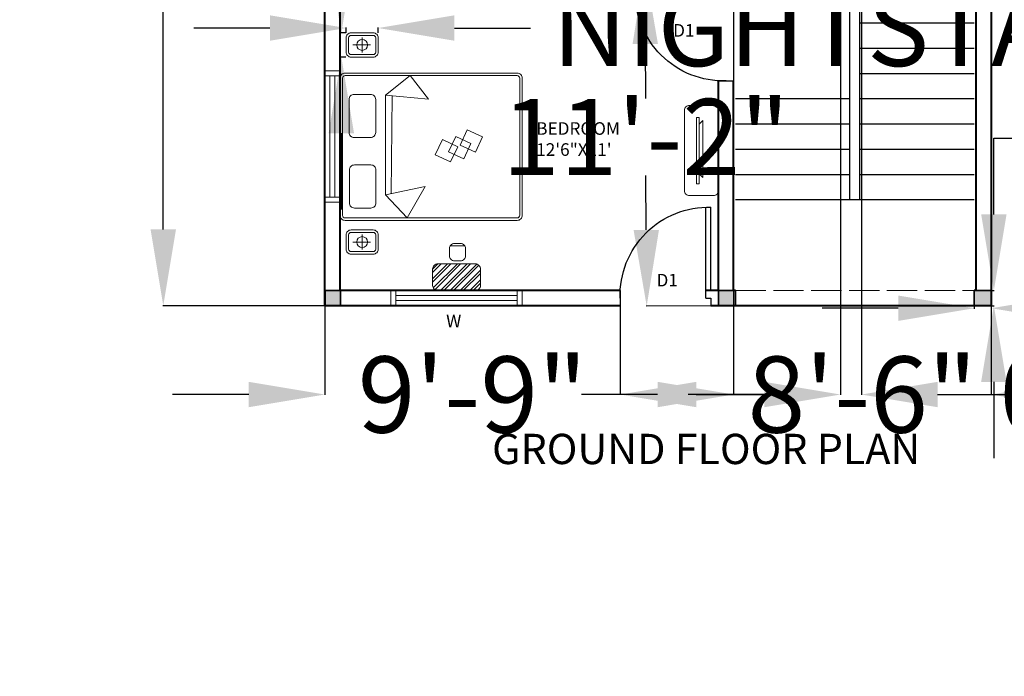
# Model space of a CAD drawing. Units: inches. Extents: x 7323 to 9737, y 2037 to 3322.
# Tile 1 of 19: x 8530 to 8921, y 2037 to 2297. Entities that reach past the tile are written whole.
import ezdxf

# ---------------------------------------------------------------- set-up
doc = ezdxf.new("R2010")
doc.units = ezdxf.units.IN
doc.header["$MEASUREMENT"] = 0
doc.linetypes.add('ACAD_ISO02W100', pattern=[15, 12, -3])
for name, color, linetype, lineweight in [('A-ANNO-DIMS', 2, 'Continuous', 18), ('A-ANNO-TEXT', 7, 'Continuous', 25), ('A-AREA-IDEN', 7, 'Continuous', 18), ('A-COLS', 1, 'Continuous', 35), ('A-DOOR', 4, 'Continuous', 25), ('A-FLOR-STRS', 7, 'Continuous', 25), ('A-FLOR-STRS-HIDN', 7, 'ACAD_ISO02W100', 18), ('A-FURN', 8, 'Continuous', 18), ('A-FURN-PATT', 252, 'Continuous', 13), ('A-GLAZ', 4, 'Continuous', 18), ('A-WALL', 7, 'Continuous', 40)]:
    doc.layers.add(name, color=color, linetype=linetype, lineweight=lineweight)
doc.layers.add('A-COLS-PATT', color=18, linetype='Continuous', lineweight=13, true_color=0x000000)
doc.styles.get("Standard").update_dxf_attribs({"font": 'arial.ttf'})
doc.dimstyles.get("Standard").update_dxf_attribs({"dimtxt": 30.18, "dimasz": 30.18, "dimexe": 0.18, "dimexo": 0.0625, "dimgap": 0.09, "dimtad": 0, "dimtih": 1, "dimtoh": 1, "dimdec": 0, "dimzin": 0, "dimdsep": 46, "dimlunit": 3, "dimtxsty": 'Standard', "dimcen": 0.09, "dimadec": 0, "dimazin": 0, "dimtfac": 1, "dimtdec": 0, "dimtofl": 0, "dimtmove": 0, "dimatfit": 3, "dimfxl": 1, "dimtolj": 1, "dimtzin": 0, "dimarcsym": 0})

# ---------------------------------------------------------------- blocks, each defined once
blk = doc.blocks.new('WIN-48')
for p, q in [((0, 0), (0, 6)), ((2, 0), (2, 6)), ((2, 4), (50, 4)), ((50, 0), (50, 6)), ((52, 0), (52, 6)), ((2, 2), (50, 2))]:
    blk.add_line(p, q)
blk = doc.blocks.new('STAIR-RETURN-FLIGHT')
for p, q in [((45.32, 110), (94.63, 110)), ((45.32, 0), (45.32, 110)), ((49.32, 0), (49.32, 110)), ((49.32, 100), (94.63, 100)), ((49.32, 90), (94.63, 90)), ((49.32, 80), (94.63, 80)), ((49.32, 70), (94.63, 70)), ((49.32, 60), (94.63, 60)), ((49.32, 50), (94.63, 50)), ((0, 40), (45.32, 40)), ((49.32, 40), (94.63, 40)), ((0, 30), (45.32, 30)), ((49.32, 30), (94.63, 30)), ((0, 20), (45.32, 20)), ((49.32, 20), (94.63, 20)), ((0, 10), (45.32, 10)), ((49.32, 10), (94.63, 10)), ((0, 0), (94.63, 0))]:
    blk.add_line(p, q)
blk = doc.blocks.new('DOOR-36')
for p, q in [((33.01, 39), (39.01, 39)), ((36.01, 5), (0.01, 5)), ((36.01, 5), (36.01, 3)), ((33.01, 3), (0.01, 3)), ((36.01, 3), (39.01, 3)), ((33.01, 0), (39.01, 0))]:
    blk.add_line(p, q)
blk.add_arc((35.01, 4), 35.01, 88.3634, 181.6366)
blk = doc.blocks.new('MEDIA-CONSOLE')
for p, q in [((5.81, 28.29), (7.29, 29.79)), ((7.29, 29.79), (7.29, 7.16)), ((7.29, 7.16), (5.81, 8.58))]:
    blk.add_line(p, q)
blk.add_lwpolyline([(13.51, 33.75, 0.414214), (11.51, 35.75), (2, 35.75, 0.414214), (0, 33.75), (0, 2, 0.414214), (2, 0), (11.51, 0, 0.414214), (13.51, 2)], format="xyb", close=True)
blk.add_lwpolyline([(5.81, 30.96), (5.81, 30.96), (4.8, 30.96), (4.8, 30.96), (4.8, 4.61), (4.8, 4.61), (5.81, 4.61), (5.81, 4.61)], close=True)
blk = doc.blocks.new('NIGHTSTAND-COMPACT')
for p, q in [((2.65, 4.81), (9.72, 4.81)), ((6.36, 7.75), (6.36, 1.85))]:
    blk.add_line(p, q)
for points in [[(0, 7.61, -0.414214), (2, 9.61), (10.71, 9.61, -0.414214), (12.71, 7.61), (12.71, 2, -0.414214), (10.71, 0), (2, 0, -0.414214), (0, 2)], [(1, 7.61, -0.414214), (2, 8.61), (10.71, 8.61, -0.414214), (11.71, 7.61), (11.71, 2, -0.414214), (10.71, 1), (2, 1, -0.414214), (1, 2)]]:
    blk.add_lwpolyline(points, format="xyb", close=True)
blk.add_circle((6.36, 4.81), 2.16)
blk = doc.blocks.new('COL-PLAN-6IN')
blk.add_lwpolyline([(0, 6), (0, 6), (6.06, 6), (6.06, 6), (6.06, 0), (6.06, 0), (0, 0), (0, 0)], close=True)
blk = doc.blocks.new('COL-STAIR-END')
blk.add_lwpolyline([(0, 6), (6.74, 6), (6.74, 0), (0, 0)], close=True)
blk = doc.blocks.new('*D43')
at = {"layer": 'A-ANNO-DIMS', "color": 0, "lineweight": -2, "transparency": 16777216}
for p, q in [((9108.94, 2438.75), (9108.94, 2468.93)), ((9104.01, 2408.57), (9109.12, 2408.57)), ((9104.01, 2375.3), (9109.12, 2375.3)), ((9108.94, 2345.12), (9108.94, 2314.94))]:
    blk.add_line(p, q, dxfattribs=at)
at = {"layer": 'A-ANNO-DIMS', "color": 0, "transparency": 16777216}
for points in [[(9103.91, 2438.75), (9113.97, 2438.75), (9108.94, 2408.57)], [(9103.91, 2345.12), (9113.97, 2345.12), (9108.94, 2375.3)]]:
    blk.add_solid(points, dxfattribs=at)
at = {"layer": 'Defpoints', "color": 0, "transparency": 16777216}
for p in [(9103.95, 2408.57), (9108.94, 2408.57), (9103.95, 2375.3)]:
    blk.add_point(p, dxfattribs=at)
at = {"layer": 'A-ANNO-DIMS', "color": 0, "transparency": 16777216, "insert": (9108.94, 2391.93), "char_height": 30.18, "attachment_point": 5}
blk.add_mtext('\\A1;BATH DOOR 2\'-9 1/2" TYP.', dxfattribs=at)
blk = doc.blocks.new('*D49')
at = {"layer": 'A-ANNO-DIMS', "color": 0, "lineweight": -2, "transparency": 16777216}
for p, q in [((8878.59, 2182.85), (8848.41, 2182.85)), ((8908.77, 2183.8), (8908.77, 2182.67)), ((8915.5, 2183.8), (8915.5, 2182.67)), ((8945.68, 2182.85), (8975.86, 2182.85))]:
    blk.add_line(p, q, dxfattribs=at)
at = {"layer": 'A-ANNO-DIMS', "color": 0, "transparency": 16777216}
for points in [[(8878.59, 2187.88), (8878.59, 2177.82), (8908.77, 2182.85)], [(8945.68, 2187.88), (8945.68, 2177.82), (8915.5, 2182.85)]]:
    blk.add_solid(points, dxfattribs=at)
at = {"layer": 'Defpoints', "color": 0, "transparency": 16777216}
for p in [(8908.77, 2183.86), (8915.5, 2183.86), (8915.5, 2182.85)]:
    blk.add_point(p, dxfattribs=at)
at = {"layer": 'A-ANNO-DIMS', "color": 0, "transparency": 16777216, "insert": (9284.58, 2182.85), "char_height": 30.18, "attachment_point": 5}
blk.add_mtext('\\A1;STAIR END POST 0\'-6 1/2" TYP.', dxfattribs=at)
blk = doc.blocks.new('*D50')
at = {"layer": 'A-ANNO-DIMS', "color": 0, "lineweight": -2, "transparency": 16777216}
for p, q in [((8916.51, 2220.04), (8916.51, 2250.22)), ((8916.51, 2250.22), (8946.69, 2250.22)), ((8915.57, 2189.86), (8916.69, 2189.86)), ((8915.57, 2183.86), (8916.69, 2183.86)), ((8916.51, 2153.68), (8916.51, 2123.5))]:
    blk.add_line(p, q, dxfattribs=at)
at = {"layer": 'A-ANNO-DIMS', "color": 0, "transparency": 16777216}
for points in [[(8911.48, 2220.04), (8921.54, 2220.04), (8916.51, 2189.86)], [(8911.48, 2153.68), (8921.54, 2153.68), (8916.51, 2183.86)]]:
    blk.add_solid(points, dxfattribs=at)
at = {"layer": 'Defpoints', "color": 0, "transparency": 16777216}
for p in [(8915.5, 2189.86), (8916.51, 2189.86), (8915.5, 2183.86)]:
    blk.add_point(p, dxfattribs=at)
at = {"layer": 'A-ANNO-DIMS', "color": 0, "transparency": 16777216, "insert": (9038.77, 2250.22), "char_height": 30.18, "attachment_point": 5}
blk.add_mtext('\\A1;0\'-6" TYP.', dxfattribs=at)
blk = doc.blocks.new('*D75')
at = {"layer": 'A-ANNO-DIMS', "color": 0, "lineweight": -2, "transparency": 16777216}
for p, q in [((8629.63, 2293.84), (8599.45, 2293.84)), ((8659.81, 2292), (8659.81, 2294.02)), ((8672.52, 2292), (8672.52, 2294.02)), ((8702.7, 2293.84), (8732.88, 2293.84))]:
    blk.add_line(p, q, dxfattribs=at)
at = {"layer": 'A-ANNO-DIMS', "color": 0, "transparency": 16777216}
for points in [[(8629.63, 2298.87), (8629.63, 2288.81), (8659.81, 2293.84)], [(8702.7, 2298.87), (8702.7, 2288.81), (8672.52, 2293.84)]]:
    blk.add_solid(points, dxfattribs=at)
at = {"layer": 'Defpoints', "color": 0, "transparency": 16777216}
for p in [(8659.81, 2291.93), (8672.52, 2293.84), (8672.52, 2291.93)]:
    blk.add_point(p, dxfattribs=at)
at = {"layer": 'A-ANNO-DIMS', "color": 0, "transparency": 16777216, "insert": (9002.27, 2293.84), "char_height": 30.18, "attachment_point": 5}
blk.add_mtext('\\A1;NIGHTSTAND 1\'-0 1/2" TYP.', dxfattribs=at)
blk = doc.blocks.new('*D76')
at = {"layer": 'A-ANNO-DIMS', "color": 0, "lineweight": -2, "transparency": 16777216}
for p, q in [((8657.91, 2322.11), (8657.91, 2352.29)), ((8657.91, 2352.29), (8688.09, 2352.29)), ((8659.75, 2291.93), (8657.73, 2291.93)), ((8659.75, 2282.32), (8657.73, 2282.32)), ((8657.91, 2252.14), (8657.91, 2221.96))]:
    blk.add_line(p, q, dxfattribs=at)
at = {"layer": 'A-ANNO-DIMS', "color": 0, "transparency": 16777216}
for points in [[(8652.88, 2322.11), (8662.94, 2322.11), (8657.91, 2291.93)], [(8652.88, 2252.14), (8662.94, 2252.14), (8657.91, 2282.32)]]:
    blk.add_solid(points, dxfattribs=at)
at = {"layer": 'Defpoints', "color": 0, "transparency": 16777216}
for p in [(8657.91, 2291.93), (8659.81, 2291.93), (8659.81, 2282.32)]:
    blk.add_point(p, dxfattribs=at)
at = {"layer": 'A-ANNO-DIMS', "color": 0, "transparency": 16777216, "insert": (8815.32, 2352.29), "char_height": 30.18, "attachment_point": 5}
blk.add_mtext('\\A1;0\'-9 1/2" TYP.', dxfattribs=at)
blk = doc.blocks.new('*D79')
at = {"layer": 'A-ANNO-DIMS', "color": 0, "lineweight": -2, "transparency": 16777216}
for p, q in [((8871.1, 2395.97), (8871.1, 2394.46)), ((8880.36, 2395.97), (8880.36, 2394.46)), ((8840.92, 2394.64), (8810.74, 2394.64)), ((8910.54, 2394.64), (8940.72, 2394.64))]:
    blk.add_line(p, q, dxfattribs=at)
at = {"layer": 'A-ANNO-DIMS', "color": 0, "transparency": 16777216}
for points in [[(8840.92, 2399.67), (8840.92, 2389.61), (8871.1, 2394.64)], [(8910.54, 2399.67), (8910.54, 2389.61), (8880.36, 2394.64)]]:
    blk.add_solid(points, dxfattribs=at)
at = {"layer": 'Defpoints', "color": 0, "transparency": 16777216}
for p in [(8871.1, 2396.03), (8880.36, 2396.03), (8880.36, 2394.64)]:
    blk.add_point(p, dxfattribs=at)
at = {"layer": 'A-ANNO-DIMS', "color": 0, "transparency": 16777216, "insert": (9195.57, 2394.64), "char_height": 30.18, "attachment_point": 5}
blk.add_mtext('\\A1;SIDE TABLE 0\'-9 1/2" TYP.', dxfattribs=at)
blk = doc.blocks.new('*D81')
at = {"layer": 'A-ANNO-DIMS', "color": 0, "lineweight": -2, "transparency": 16777216}
for p, q in [((8651.33, 2671.86), (8587.16, 2671.86)), ((8587.34, 2641.68), (8587.34, 2443.36)), ((8587.34, 2214.04), (8587.34, 2412.36)), ((8651.33, 2183.86), (8587.16, 2183.86))]:
    blk.add_line(p, q, dxfattribs=at)
at = {"layer": 'A-ANNO-DIMS', "color": 0, "transparency": 16777216}
for points in [[(8582.31, 2641.68), (8592.37, 2641.68), (8587.34, 2671.86)], [(8582.31, 2214.04), (8592.37, 2214.04), (8587.34, 2183.86)]]:
    blk.add_solid(points, dxfattribs=at)
at = {"layer": 'Defpoints', "color": 0, "transparency": 16777216}
for p in [(8587.34, 2671.86), (8651.39, 2671.86), (8651.39, 2183.86)]:
    blk.add_point(p, dxfattribs=at)
at = {"layer": 'A-ANNO-DIMS', "color": 0, "transparency": 16777216, "insert": (8587.34, 2427.86), "char_height": 30.18, "attachment_point": 5}
blk.add_mtext('\\A1;40\'-8"', dxfattribs=at)
blk = doc.blocks.new('*D97')
at = {"layer": 'A-ANNO-DIMS', "color": 0, "lineweight": -2, "transparency": 16777216}
for p, q in [((8813.39277, 2308.800309), (8813.39277, 2148.482809)), ((8915.39277, 2183.800309), (8915.39277, 2148.482809)), ((8783.21277, 2148.662809), (8753.03277, 2148.662809)), ((8945.57277, 2148.662809), (8975.75277, 2148.662809))]:
    blk.add_line(p, q, dxfattribs=at)
at = {"layer": 'A-ANNO-DIMS', "color": 0, "transparency": 16777216}
for points in [[(8783.21277, 2153.692809), (8783.21277, 2143.632809), (8813.39277, 2148.662809)], [(8945.57277, 2153.692809), (8945.57277, 2143.632809), (8915.39277, 2148.662809)]]:
    blk.add_solid(points, dxfattribs=at)
at = {"layer": 'Defpoints', "color": 0, "transparency": 16777216}
for p in [(8813.39277, 2308.862809), (8915.39277, 2183.862809), (8915.39277, 2148.662809)]:
    blk.add_point(p, dxfattribs=at)
at = {"layer": 'A-ANNO-DIMS', "color": 0, "transparency": 16777216, "insert": (8864.39277, 2148.662809), "char_height": 30.18, "attachment_point": 5}
blk.add_mtext('\\A1;8\'-6"', dxfattribs=at)
blk = doc.blocks.new('*D98')
at = {"layer": 'A-ANNO-DIMS', "color": 0, "lineweight": -2, "transparency": 16777216}
for p, q in [((8813.33, 2317.86), (8778.01, 2317.67)), ((8778.36, 2287.49), (8778.48, 2265.91)), ((8778.77, 2213.85), (8778.65, 2235.43)), ((8814.07, 2183.86), (8778.75, 2183.67))]:
    blk.add_line(p, q, dxfattribs=at)
at = {"layer": 'A-ANNO-DIMS', "color": 0, "transparency": 16777216}
for points in [[(8783.39, 2287.52), (8773.33, 2287.46), (8778.19, 2317.67)], [(8783.79, 2213.88), (8773.74, 2213.82), (8778.93, 2183.67)]]:
    blk.add_solid(points, dxfattribs=at)
at = {"layer": 'Defpoints', "color": 0, "transparency": 16777216}
for p in [(8778.19, 2317.67), (8813.39, 2317.86), (8814.13, 2183.86)]:
    blk.add_point(p, dxfattribs=at)
at = {"layer": 'A-ANNO-DIMS', "color": 0, "transparency": 16777216, "insert": (8778.56, 2250.67), "char_height": 30.18, "attachment_point": 5}
blk.add_mtext('\\A1;11\'-2"', dxfattribs=at)
blk = doc.blocks.new('*D107')
at = {"layer": 'A-ANNO-DIMS', "color": 0, "lineweight": -2, "transparency": 16777216}
for p, q in [((8855.74, 2420.27), (8855.74, 2148.48)), ((8864.06, 2412.89), (8864.06, 2148.48)), ((8825.56, 2148.66), (8795.38, 2148.66)), ((8894.24, 2148.66), (8924.42, 2148.66))]:
    blk.add_line(p, q, dxfattribs=at)
at = {"layer": 'A-ANNO-DIMS', "color": 0, "transparency": 16777216}
for points in [[(8825.56, 2153.69), (8825.56, 2143.63), (8855.74, 2148.66)], [(8894.24, 2153.69), (8894.24, 2143.63), (8864.06, 2148.66)]]:
    blk.add_solid(points, dxfattribs=at)
at = {"layer": 'Defpoints', "color": 0, "transparency": 16777216}
for p in [(8855.74, 2420.33), (8864.06, 2412.95), (8864.06, 2148.66)]:
    blk.add_point(p, dxfattribs=at)
at = {"layer": 'A-ANNO-DIMS', "color": 0, "transparency": 16777216, "insert": (8999.78, 2148.66), "char_height": 30.18, "attachment_point": 5}
blk.add_mtext('\\A1;0\'-8 1/2"', dxfattribs=at)
blk = doc.blocks.new('*D113')
at = {"layer": 'A-ANNO-DIMS', "color": 0, "lineweight": -2, "transparency": 16777216}
for p, q in [((8651.39277, 2183.800309), (8651.39277, 2148.482809)), ((8768.39277, 2183.800309), (8768.39277, 2148.482809)), ((8621.21277, 2148.662809), (8591.03277, 2148.662809)), ((8798.57277, 2148.662809), (8828.75277, 2148.662809))]:
    blk.add_line(p, q, dxfattribs=at)
at = {"layer": 'A-ANNO-DIMS', "color": 0, "transparency": 16777216}
for points in [[(8621.21277, 2153.692809), (8621.21277, 2143.632809), (8651.39277, 2148.662809)], [(8798.57277, 2153.692809), (8798.57277, 2143.632809), (8768.39277, 2148.662809)]]:
    blk.add_solid(points, dxfattribs=at)
at = {"layer": 'Defpoints', "color": 0, "transparency": 16777216}
for p in [(8651.39277, 2183.862809), (8768.39277, 2183.862809), (8768.39277, 2148.662809)]:
    blk.add_point(p, dxfattribs=at)
at = {"layer": 'A-ANNO-DIMS', "color": 0, "transparency": 16777216, "insert": (8709.89277, 2148.662809), "char_height": 30.18, "attachment_point": 5}
blk.add_mtext('\\A1;9\'-9"', dxfattribs=at)

msp = doc.modelspace()

# ---------------------------------------------------------------- hatches: boundary and pattern name
at = {"layer": 'A-COLS-PATT'}
h = msp.add_hatch(color=256, dxfattribs=at)
h.dxf.hatch_style = 1
h.paths.add_polyline_path([(8915.39, 2189.86), (8908.77, 2189.86), (8908.77, 2183.86), (8915.39, 2183.86)])
h.paths.add_polyline_path([(8657.61, 2189.86), (8651.55, 2189.86), (8651.55, 2183.86), (8657.61, 2183.86)])
h.paths.add_polyline_path([(8814.13, 2189.86), (8807.39, 2189.86), (8807.39, 2183.86), (8814.13, 2183.86)])
h.paths.add_polyline_path([(8813.39, 2317.86), (8807.36, 2317.86), (8807.36, 2311.86), (8813.39, 2311.86)])
h.paths.add_polyline_path([(8915.34, 2313.13), (8909.39, 2313.13), (8909.39, 2307.13), (8915.34, 2307.13)])
h.paths.add_polyline_path([(8657.62, 2317.86), (8657.39, 2317.86), (8657.39, 2318.08), (8651.55, 2318.08), (8651.55, 2312.08), (8657.62, 2312.08)])
h.paths.add_polyline_path([(8915.39, 2671.84), (8909.37, 2671.84), (8909.37, 2665.86), (8909.39, 2665.86), (8915.39, 2665.84)])
h.paths.add_polyline_path([(8657.59, 2671.81), (8651.52, 2671.81), (8651.52, 2665.81), (8657.39, 2665.81), (8657.39, 2665.86)])
h.paths.add_polyline_path([(8915.28, 2503.94), (8909.39, 2503.94), (8909.39, 2503.86), (8909.22, 2497.94), (8915.28, 2497.94)])
h.paths.add_polyline_path([(8657.53, 2503.86), (8657.39, 2503.86), (8651.46, 2503.96), (8651.46, 2497.96), (8657.53, 2497.96)])
h.paths.add_polyline_path([(9014.24, 2519.3), (9013.95, 2519.3), (9008.18, 2519.31), (9008.18, 2513.31), (9014.24, 2513.31)])
h.paths.add_polyline_path([(9013.95, 2687.3), (9007.95, 2687.3), (9007.95, 2681.3), (9013.95, 2681.3)])
h.paths.add_polyline_path([(9271.95, 2687.3), (9266.01, 2687.3), (9266.01, 2681.35), (9271.95, 2681.35)])
h.paths.add_polyline_path([(9271.95, 2205.3), (9265.32, 2205.3), (9265.32, 2199.3), (9271.95, 2199.3)])
h.paths.add_polyline_path([(9170.68, 2205.3), (9163.95, 2205.3), (9163.95, 2199.3), (9170.68, 2199.3)])
h.paths.add_polyline_path([(9013.95, 2205.3), (9007.95, 2205.3), (9007.95, 2199.3), (9013.95, 2199.3)])
h.paths.add_polyline_path([(9271.95, 2519.51), (9265.95, 2519.51), (9265.95, 2519.3), (9265.93, 2513.51), (9271.95, 2513.51)])
h.paths.add_polyline_path([(9271.95, 2328.64), (9265.95, 2328.64), (9265.95, 2322.64), (9271.95, 2322.64)])
h.paths.add_polyline_path([(9014.35, 2333.3), (9013.95, 2333.3), (9013.95, 2333.58), (9008.29, 2333.58), (9008.29, 2327.58), (9014.35, 2327.58)])
at = {"layer": 'A-FURN-PATT'}
h = msp.add_hatch(dxfattribs=at)
h.set_pattern_fill('ANSI32', color=256, scale=7.3, angle=180)
h.set_pattern_definition([(225, (15955.0248, 4971.0192), (1.9357048, -1.9357048), []), (225, (15953.7343, 4971.0192), (1.9357048, -1.9357048), [])])
h.paths.add_polyline_path([(8711.04, 2189.86, 0.414214), (8713.04, 2191.86), (8713.04, 2198.41, 0.414214), (8711.04, 2200.41), (8696.09, 2200.41, 0.414214), (8694.09, 2198.41), (8694.09, 2191.86, 0.414214), (8696.09, 2189.86)])

# ---------------------------------------------------------------- linework, layer by layer
at = {"layer": 'A-FLOR-STRS-HIDN'}
msp.add_line((8814.13, 2189.86), (8908.77, 2189.86), dxfattribs=at)
at = {"layer": 'A-FURN'}
for p, q in [((8675.43, 2267.3), (8685.14, 2274.98)), ((8685.14, 2274.98), (8692.48, 2265.69)), ((8675.43, 2267.3), (8675.43, 2227.78)), ((8692.48, 2265.69), (8675.43, 2267.3)), ((8678.06, 2267.05), (8677.69, 2228.26)), ((8691.17, 2231.1), (8675.43, 2227.78)), ((8683.98, 2218.64), (8691.17, 2231.1)), ((8675.43, 2227.78), (8683.98, 2218.64)), ((8706.83, 2207.56), (8701.12, 2207.56))]:
    msp.add_line(p, q, dxfattribs=at)
for points in [[(8657.39, 2219.64, 0.414214), (8659.39, 2217.64), (8727.59, 2217.64, 0.414214), (8729.59, 2219.64), (8729.59, 2273.98, 0.414214), (8727.59, 2275.98), (8659.39, 2275.98, 0.414214), (8657.39, 2273.98)], [(8658.39, 2219.64, 0.414214), (8659.39, 2218.64), (8727.59, 2218.64, 0.414214), (8728.59, 2219.64), (8728.59, 2273.98, 0.414214), (8727.59, 2274.98), (8659.39, 2274.98, 0.414214), (8658.39, 2273.98)], [(8660.98, 2265.57, -0.414214), (8662.98, 2267.57), (8669.53, 2267.57, -0.414214), (8671.53, 2265.57), (8671.53, 2252.48, -0.414214), (8669.53, 2250.48), (8662.98, 2250.48, -0.414214), (8660.98, 2252.48)], [(8661.09, 2237.62, -0.414214), (8663.09, 2239.62), (8669.64, 2239.62, -0.414214), (8671.64, 2237.62), (8671.64, 2224.54, -0.414214), (8669.64, 2222.54), (8663.09, 2222.54, -0.414214), (8661.09, 2224.54)], [(8707.16, 2203.63, -0.414214), (8705.16, 2201.63), (8702.72, 2201.63, -0.414214), (8700.72, 2203.63), (8700.72, 2206.47, -0.414214), (8702.72, 2208.47), (8705.16, 2208.47, -0.414214), (8707.16, 2206.47)], [(8713.04, 2191.86, -0.414214), (8711.04, 2189.86), (8696.09, 2189.86, -0.414214), (8694.09, 2191.86), (8694.09, 2198.41, -0.414214), (8696.09, 2200.41), (8711.04, 2200.41, -0.414214), (8713.04, 2198.41)]]:
    msp.add_lwpolyline(points, format="xyb", close=True, dxfattribs=at)
for points in [[(8707.81, 2253.54), (8704.96, 2247.49), (8711.02, 2244.64), (8713.86, 2250.69)], [(8697.96, 2249.68), (8695.12, 2243.62), (8701.17, 2240.78), (8704.02, 2246.83)], [(8703.23, 2250.9), (8700.38, 2244.84), (8706.44, 2242), (8709.29, 2248.05)]]:
    msp.add_lwpolyline(points, close=True, dxfattribs=at)
at = {"layer": 'A-WALL'}
for p, q in [((8651.39, 2183.86), (8651.39, 2671.86)), ((8915.39, 2671.86), (8915.39, 2183.86)), ((8909.39, 2497.86), (8909.39, 2189.86)), ((8657.39, 2189.86), (8657.39, 2311.86)), ((8807.39, 2189.86), (8807.39, 2272.91)), ((8813.39, 2189.86), (8813.39, 2272.86)), ((8768.44, 2189.86), (8657.39, 2189.86)), ((8807.39, 2189.86), (8802.39, 2189.86)), ((8814.13, 2189.86), (8813.39, 2189.86)), ((8909.39, 2189.86), (8908.77, 2189.86)), ((8768.39, 2183.86), (8651.39, 2183.86)), ((8915.39, 2183.86), (8804.39, 2183.86))]:
    msp.add_line(p, q, dxfattribs=at)

# ---------------------------------------------------------------- block references
at = {"layer": 'A-COLS'}
for name, p in [('COL-PLAN-6IN', (8651.55, 2183.86)), ('COL-STAIR-END', (8807.39, 2183.86)), ('COL-STAIR-END', (8908.77, 2183.86))]:
    msp.add_blockref(name, p, dxfattribs=at)
at = {"layer": 'A-DOOR', "extrusion": (0, 0, -1), "zscale": -1}
for p, rotation in [((-8774.38, 2311.86), 180), ((-8807.39, 2222.88), 269.9999999999935)]:
    msp.add_blockref('DOOR-36', p, dxfattribs=dict(at, rotation=rotation))
at = {"layer": 'A-FLOR-STRS'}
msp.add_blockref('STAIR-RETURN-FLIGHT', (8814.13, 2225.86), dxfattribs=at)
at = {"layer": 'A-FURN'}
for name, p in [('NIGHTSTAND-COMPACT', (8659.81, 2282.32)), ('MEDIA-CONSOLE', (8793.88, 2227.46)), ('NIGHTSTAND-COMPACT', (8659.81, 2204.26))]:
    msp.add_blockref(name, p, dxfattribs=at)
at = {"layer": 'A-GLAZ', "rotation": 89.99999999999191}
msp.add_blockref('WIN-48', (8657.39, 2224.86), dxfattribs=at)
at = {"layer": 'A-GLAZ'}
msp.add_blockref('WIN-48', (8677.56, 2183.86), dxfattribs=at)

# ---------------------------------------------------------------- texts
at = {"layer": 'A-ANNO-TEXT', "attachment_point": 1}
for s, width, insert, char_height in [('D1', 26.304, (8789.41, 2295.4), 5), ('D1', 26.304, (8782.82, 2196.47), 5), ('W', 26.304, (8699.46, 2180.27), 5), ('GROUND FLOOR PLAN', 222.6475, (8717.65, 2133.1), 12)]:
    msp.add_mtext_dynamic_manual_height_columns(s, width=width, gutter_width=1, heights=[0], dxfattribs=dict(at, insert=insert, char_height=char_height))
at = {"layer": 'A-AREA-IDEN', "insert": (8735.14, 2256.54), "char_height": 5, "attachment_point": 1}
msp.add_mtext_dynamic_manual_height_columns('BEDROOM\\P12\'6"X11\'', width=44.1759, gutter_width=1, heights=[0], dxfattribs=at)

# ---------------------------------------------------------------- dimensions: what is measured, and where the dimension line sits
at = {"layer": 'A-ANNO-DIMS'}
for base, p1, p2, angle, picture, middle in [((8587.34, 2671.86), (8651.39, 2183.86), (8651.39, 2671.86), 90, '*D81', (8587.34, 2427.86)), ((8778.19, 2317.67), (8814.13, 2183.86), (8813.39, 2317.86), 90.3155, '*D98', (8778.56, 2250.67))]:
    dim = msp.add_linear_dim(base=base, p1=p1, p2=p2, angle=angle, dimstyle='Standard', override={"dimdec": 1, "dimlfac": 1, "dimrnd": 0, "dimzin": 1, "dimdsep": 46, "dimlunit": 4, "dimfrac": 2}, dxfattribs=at)
    dim.commit()
    dim.dimension.update_dxf_attribs({"geometry": picture, "text_midpoint": middle})
for base, p1, p2, text, picture, middle in [((8880.36, 2394.64), (8871.1, 2396.03), (8880.36, 2396.03), 'SIDE TABLE <> TYP.', '*D79', (9195.57, 2394.64)), ((8672.52, 2293.84), (8659.81, 2291.93), (8672.52, 2291.93), 'NIGHTSTAND <> TYP.', '*D75', (9002.27, 2293.84)), ((8915.5, 2182.85), (8908.77, 2183.86), (8915.5, 2183.86), 'STAIR END POST <> TYP.', '*D49', (9284.58, 2182.85))]:
    dim = msp.add_linear_dim(base=base, p1=p1, p2=p2, text=text, dimstyle='Standard', override={"dimdec": 1, "dimlfac": 1, "dimrnd": 0, "dimzin": 1, "dimdsep": 46, "dimlunit": 4, "dimfrac": 2}, dxfattribs=at)
    dim.commit()
    dim.dimension.update_dxf_attribs({"geometry": picture, "text_midpoint": middle})
for base, p1, p2, text, picture, middle in [((9108.94, 2408.57), (9103.95, 2375.3), (9103.95, 2408.57), 'BATH DOOR <> TYP.', '*D43', (9108.94, 2391.93)), ((8657.91, 2291.93), (8659.81, 2282.32), (8659.81, 2291.93), '<> TYP.', '*D76', (8815.32, 2352.29)), ((8916.51, 2189.86), (8915.5, 2183.86), (8915.5, 2189.86), '<> TYP.', '*D50', (9038.77, 2250.22))]:
    dim = msp.add_linear_dim(base=base, p1=p1, p2=p2, angle=90, text=text, dimstyle='Standard', override={"dimdec": 1, "dimlfac": 1, "dimrnd": 0, "dimzin": 1, "dimdsep": 46, "dimlunit": 4, "dimfrac": 2}, dxfattribs=at)
    dim.commit()
    dim.dimension.update_dxf_attribs({"geometry": picture, "text_midpoint": middle})
for base, p1, p2, picture, middle in [((8864.06, 2148.66), (8855.74, 2420.33), (8864.06, 2412.95), '*D107', (8999.78, 2148.66)), ((8915.39, 2148.66), (8813.39, 2308.86), (8915.39, 2183.86), '*D97', (8864.39, 2148.66)), ((8768.39, 2148.66), (8651.39, 2183.86), (8768.39, 2183.86), '*D113', (8709.89, 2148.66))]:
    dim = msp.add_linear_dim(base=base, p1=p1, p2=p2, dimstyle='Standard', override={"dimdec": 1, "dimlfac": 1, "dimrnd": 0, "dimzin": 1, "dimdsep": 46, "dimlunit": 4, "dimfrac": 2}, dxfattribs=at)
    dim.commit()
    dim.dimension.update_dxf_attribs({"geometry": picture, "text_midpoint": middle})

doc.saveas('drawing.dxf')
